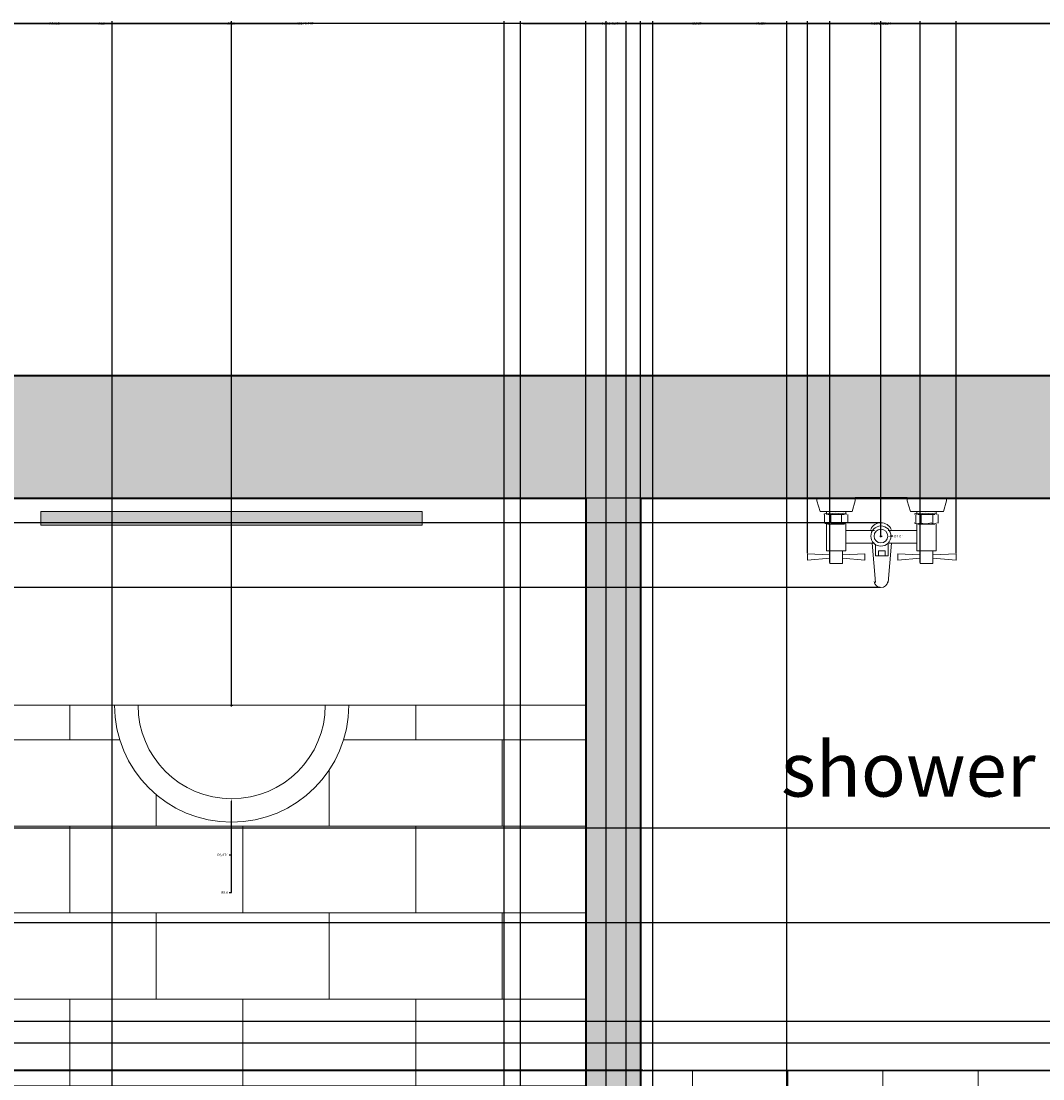
# Model space of a CAD drawing. Units: inches. Extents: x 6 to 575, y 34 to 566.
# Tile 9 of 21: x 76 to 151, y 488 to 566. Entities that reach past the tile are written whole.
import ezdxf

# ---------------------------------------------------------------- set-up
doc = ezdxf.new("R2010")
doc.units = ezdxf.units.IN
for name, color, linetype, lineweight in [('A-ANNO-DIMS', 2, 'Continuous', 18), ('A-ANNO-TEXT', 6, 'Continuous', 18), ('A-FLOR-CASE', 2, 'Continuous', 18), ('A-FLOR-CASE-PATT', 2, 'Continuous', 9), ('A-FLOR-FIXT', 9, 'Continuous', 18), ('A-FLOR-PATT', 252, 'Continuous', 9), ('A-WALL-PATT', 251, 'Continuous', 9), ('FUR', 2, 'Continuous', 18), ('WALLS', 7, 'Continuous', 35)]:
    doc.layers.add(name, color=color, linetype=linetype, lineweight=lineweight)
doc.styles.add('PDF Arial Narrow', font='txt')
doc.styles.get("Standard").update_dxf_attribs({"font": 'arial.ttf'})
doc.dimstyles.get("Standard").update_dxf_attribs({"dimtxt": 0.18, "dimasz": 0.18, "dimexe": 0.18, "dimexo": 0.0625, "dimgap": 0.09, "dimtad": 0, "dimtih": 1, "dimtoh": 1, "dimdec": 4, "dimzin": 0, "dimdsep": 46, "dimtxsty": 'Standard', "dimcen": 0.09, "dimadec": 0, "dimazin": 0, "dimtfac": 1, "dimtdec": 4, "dimtofl": 0, "dimtmove": 0, "dimatfit": 3, "dimfxl": 1, "dimtolj": 1, "dimtzin": 0, "dimarcsym": 0})

# ---------------------------------------------------------------- blocks, each defined once
blk = doc.blocks.new('*D30')
at = {"layer": 'A-ANNO-DIMS', "color": 0, "lineweight": -2, "transparency": 16777216}
for p, q in [((32.596, 539.801), (6.649, 539.801)), ((6.829, 539.621), (6.829, 299.97)), ((6.829, 59.955), (6.829, 299.606)), ((197.625, 59.775), (6.649, 59.775))]:
    blk.add_line(p, q, dxfattribs=at)
at = {"layer": 'A-ANNO-DIMS', "color": 0, "transparency": 16777216}
for points in [[(6.799, 539.621), (6.859, 539.621), (6.829, 539.801)], [(6.799, 59.955), (6.859, 59.955), (6.829, 59.775)]]:
    blk.add_solid(points, dxfattribs=at)
at = {"layer": 'Defpoints', "color": 0, "transparency": 16777216}
for p in [(32.659, 539.801), (6.829, 59.775), (197.687, 59.775)]:
    blk.add_point(p, dxfattribs=at)
at = {"layer": 'A-ANNO-DIMS', "color": 0, "transparency": 16777216, "insert": (6.829, 299.788), "char_height": 0.18, "attachment_point": 5}
blk.add_mtext('\\A1;480', dxfattribs=at)
blk = doc.blocks.new('*D31')
at = {"layer": 'A-ANNO-DIMS', "color": 0, "lineweight": -2, "transparency": 16777216}
for p, q in [((32.659, 539.863), (32.659, 565.811)), ((32.839, 565.631), (96.378, 565.631)), ((160.479, 565.631), (96.939, 565.631)), ((160.659, 539.863), (160.659, 565.811))]:
    blk.add_line(p, q, dxfattribs=at)
at = {"layer": 'A-ANNO-DIMS', "color": 0, "transparency": 16777216}
for points in [[(32.839, 565.661), (32.839, 565.601), (32.659, 565.631)], [(160.479, 565.661), (160.479, 565.601), (160.659, 565.631)]]:
    blk.add_solid(points, dxfattribs=at)
at = {"layer": 'Defpoints', "color": 0, "transparency": 16777216}
for p in [(160.659, 565.631), (32.659, 539.801), (160.659, 539.801)]:
    blk.add_point(p, dxfattribs=at)
at = {"layer": 'A-ANNO-DIMS', "color": 0, "transparency": 16777216, "insert": (96.659, 565.631), "char_height": 0.18, "attachment_point": 5}
blk.add_mtext('\\A1;128', dxfattribs=at)
blk = doc.blocks.new('*D55')
at = {"layer": 'A-ANNO-DIMS', "color": 0, "lineweight": -2, "transparency": 16777216}
for p, q in [((41.659, 286.127), (41.659, 565.811)), ((41.839, 565.631), (81.788, 565.631)), ((122.385, 565.631), (82.436, 565.631)), ((122.565, 286.127), (122.565, 565.811))]:
    blk.add_line(p, q, dxfattribs=at)
at = {"layer": 'A-ANNO-DIMS', "color": 0, "transparency": 16777216}
for points in [[(41.839, 565.661), (41.839, 565.601), (41.659, 565.631)], [(122.385, 565.661), (122.385, 565.601), (122.565, 565.631)]]:
    blk.add_solid(points, dxfattribs=at)
at = {"layer": 'Defpoints', "color": 0, "transparency": 16777216}
for p in [(122.565, 565.631), (41.659, 286.064), (122.565, 286.064)]:
    blk.add_point(p, dxfattribs=at)
at = {"layer": 'A-ANNO-DIMS', "color": 0, "transparency": 16777216, "insert": (82.112, 565.631), "char_height": 0.18, "attachment_point": 5}
blk.add_mtext('\\A1;80.9', dxfattribs=at)
blk = doc.blocks.new('*D62')
at = {"layer": 'A-ANNO-DIMS', "color": 0, "lineweight": -2, "transparency": 16777216}
for p, q in [((117.659, 530.863), (117.659, 565.811)), ((117.839, 565.631), (119.506, 565.631)), ((121.479, 565.631), (119.811, 565.631)), ((121.659, 530.863), (121.659, 565.811))]:
    blk.add_line(p, q, dxfattribs=at)
at = {"layer": 'A-ANNO-DIMS', "color": 0, "transparency": 16777216}
for points in [[(117.839, 565.661), (117.839, 565.601), (117.659, 565.631)], [(121.479, 565.661), (121.479, 565.601), (121.659, 565.631)]]:
    blk.add_solid(points, dxfattribs=at)
at = {"layer": 'Defpoints', "color": 0, "transparency": 16777216}
for p in [(121.659, 565.631), (117.659, 530.801), (121.659, 530.801)]:
    blk.add_point(p, dxfattribs=at)
at = {"layer": 'A-ANNO-DIMS', "color": 0, "transparency": 16777216, "insert": (119.659, 565.631), "char_height": 0.18, "attachment_point": 5}
blk.add_mtext('\\A1;4', dxfattribs=at)
blk = doc.blocks.new('*D66')
at = {"layer": 'A-ANNO-DIMS', "color": 0, "lineweight": -2, "transparency": 16777216}
for p, q in [((41.659, 440.863), (41.659, 565.811)), ((41.839, 565.631), (61.878, 565.631)), ((82.712, 565.631), (62.673, 565.631)), ((82.892, 440.863), (82.892, 565.811))]:
    blk.add_line(p, q, dxfattribs=at)
at = {"layer": 'A-ANNO-DIMS', "color": 0, "transparency": 16777216}
for points in [[(41.839, 565.661), (41.839, 565.601), (41.659, 565.631)], [(82.712, 565.661), (82.712, 565.601), (82.892, 565.631)]]:
    blk.add_solid(points, dxfattribs=at)
at = {"layer": 'Defpoints', "color": 0, "transparency": 16777216}
for p in [(82.892, 565.631), (41.659, 440.801), (82.892, 440.801)]:
    blk.add_point(p, dxfattribs=at)
at = {"layer": 'A-ANNO-DIMS', "color": 0, "transparency": 16777216, "insert": (62.275, 565.631), "char_height": 0.18, "attachment_point": 5}
blk.add_mtext('\\A1;41.23', dxfattribs=at)
blk = doc.blocks.new('*D67')
at = {"layer": 'A-ANNO-DIMS', "color": 0, "lineweight": -2, "transparency": 16777216}
for p, q in [((82.892, 440.863), (82.892, 565.811)), ((83.072, 565.631), (96.81, 565.631)), ((111.479, 565.631), (97.74, 565.631)), ((111.659, 440.863), (111.659, 565.811))]:
    blk.add_line(p, q, dxfattribs=at)
at = {"layer": 'A-ANNO-DIMS', "color": 0, "transparency": 16777216}
for points in [[(83.072, 565.661), (83.072, 565.601), (82.892, 565.631)], [(111.479, 565.661), (111.479, 565.601), (111.659, 565.631)]]:
    blk.add_solid(points, dxfattribs=at)
at = {"layer": 'Defpoints', "color": 0, "transparency": 16777216}
for p in [(111.659, 565.631), (82.892, 440.801), (111.659, 440.801)]:
    blk.add_point(p, dxfattribs=at)
at = {"layer": 'A-ANNO-DIMS', "color": 0, "transparency": 16777216, "insert": (97.275, 565.631), "char_height": 0.18, "attachment_point": 5}
blk.add_mtext('\\A1;28.767', dxfattribs=at)
blk = doc.blocks.new('*D68')
at = {"layer": 'A-ANNO-DIMS', "color": 0, "lineweight": -2, "transparency": 16777216}
for p, q in [((206.596, 530.801), (6.649, 530.801)), ((6.829, 530.621), (6.829, 509.957)), ((6.829, 488.928), (6.829, 509.593)), ((248.571, 488.748), (6.649, 488.748))]:
    blk.add_line(p, q, dxfattribs=at)
at = {"layer": 'A-ANNO-DIMS', "color": 0, "transparency": 16777216}
for points in [[(6.799, 530.621), (6.859, 530.621), (6.829, 530.801)], [(6.799, 488.928), (6.859, 488.928), (6.829, 488.748)]]:
    blk.add_solid(points, dxfattribs=at)
at = {"layer": 'Defpoints', "color": 0, "transparency": 16777216}
for p in [(206.659, 530.801), (6.829, 488.748), (248.633, 488.748)]:
    blk.add_point(p, dxfattribs=at)
at = {"layer": 'A-ANNO-DIMS', "color": 0, "transparency": 16777216, "insert": (6.829, 509.775), "char_height": 0.18, "attachment_point": 5}
blk.add_mtext('\\A1;42.05', dxfattribs=at)
blk = doc.blocks.new('*D71')
at = {"layer": 'A-ANNO-DIMS', "color": 0, "lineweight": -2, "transparency": 16777216}
for p, q in [((246.62, 490.777), (6.649, 490.777)), ((6.829, 490.597), (6.829, 489.945)), ((6.829, 488.928), (6.829, 489.581)), ((248.571, 488.748), (6.649, 488.748))]:
    blk.add_line(p, q, dxfattribs=at)
at = {"layer": 'A-ANNO-DIMS', "color": 0, "transparency": 16777216}
for points in [[(6.799, 490.597), (6.859, 490.597), (6.829, 490.777)], [(6.799, 488.928), (6.859, 488.928), (6.829, 488.748)]]:
    blk.add_solid(points, dxfattribs=at)
at = {"layer": 'Defpoints', "color": 0, "transparency": 16777216}
for p in [(246.683, 490.777), (6.829, 488.748), (248.633, 488.748)]:
    blk.add_point(p, dxfattribs=at)
at = {"layer": 'A-ANNO-DIMS', "color": 0, "transparency": 16777216, "insert": (6.829, 489.763), "char_height": 0.18, "attachment_point": 5}
blk.add_mtext('\\A1;2.03', dxfattribs=at)
blk = doc.blocks.new('*D109')
at = {"layer": 'A-ANNO-DIMS', "color": 0, "lineweight": -2, "transparency": 16777216}
for p, q in [((112.851, 431.863), (112.851, 565.811)), ((113.031, 565.631), (154.931, 565.631)), ((197.479, 565.631), (155.579, 565.631)), ((197.659, 431.863), (197.659, 565.811))]:
    blk.add_line(p, q, dxfattribs=at)
at = {"layer": 'A-ANNO-DIMS', "color": 0, "transparency": 16777216}
for points in [[(113.031, 565.661), (113.031, 565.601), (112.851, 565.631)], [(197.479, 565.661), (197.479, 565.601), (197.659, 565.631)]]:
    blk.add_solid(points, dxfattribs=at)
at = {"layer": 'Defpoints', "color": 0, "transparency": 16777216}
for p in [(197.659, 565.631), (112.851, 431.801), (197.659, 431.801)]:
    blk.add_point(p, dxfattribs=at)
at = {"layer": 'A-ANNO-DIMS', "color": 0, "transparency": 16777216, "insert": (155.255, 565.631), "char_height": 0.18, "attachment_point": 5}
blk.add_mtext('\\A1;84.8', dxfattribs=at)
blk = doc.blocks.new('*D113')
at = {"layer": 'A-ANNO-DIMS', "color": 0, "lineweight": -2, "transparency": 16777216}
for p, q in [((65.649, 530.863), (65.649, 565.811)), ((65.829, 565.631), (91.278, 565.631)), ((117.479, 565.631), (92.03, 565.631)), ((117.659, 530.863), (117.659, 565.811))]:
    blk.add_line(p, q, dxfattribs=at)
at = {"layer": 'A-ANNO-DIMS', "color": 0, "transparency": 16777216}
for points in [[(65.829, 565.661), (65.829, 565.601), (65.649, 565.631)], [(117.479, 565.661), (117.479, 565.601), (117.659, 565.631)]]:
    blk.add_solid(points, dxfattribs=at)
at = {"layer": 'Defpoints', "color": 0, "transparency": 16777216}
for p in [(117.659, 565.631), (65.649, 530.801), (117.659, 530.801)]:
    blk.add_point(p, dxfattribs=at)
at = {"layer": 'A-ANNO-DIMS', "color": 0, "transparency": 16777216, "insert": (91.654, 565.631), "char_height": 0.18, "attachment_point": 5}
blk.add_mtext('\\A1;52.01', dxfattribs=at)
blk = doc.blocks.new('*D118')
at = {"layer": 'A-ANNO-DIMS', "color": 0, "lineweight": -2, "transparency": 16777216}
for p, q in [((65.649, 515.657), (65.649, 565.811)), ((65.829, 565.631), (78.186, 565.631)), ((91.474, 565.631), (79.118, 565.631)), ((91.654, 515.657), (91.654, 565.811))]:
    blk.add_line(p, q, dxfattribs=at)
at = {"layer": 'A-ANNO-DIMS', "color": 0, "transparency": 16777216}
for points in [[(65.829, 565.661), (65.829, 565.601), (65.649, 565.631)], [(91.474, 565.661), (91.474, 565.601), (91.654, 565.631)]]:
    blk.add_solid(points, dxfattribs=at)
at = {"layer": 'Defpoints', "color": 0, "transparency": 16777216}
for p in [(91.654, 565.631), (65.649, 515.594), (91.654, 515.594)]:
    blk.add_point(p, dxfattribs=at)
at = {"layer": 'A-ANNO-DIMS', "color": 0, "transparency": 16777216, "insert": (78.652, 565.631), "char_height": 0.18, "attachment_point": 5}
blk.add_mtext('\\A1;26.005', dxfattribs=at)
blk = doc.blocks.new('*D175')
at = {"layer": 'A-ANNO-DIMS', "color": 0, "lineweight": -2, "transparency": 16777216}
for p, q in [((121.659, 530.863), (121.659, 565.811)), ((121.839, 565.631), (139.387, 565.631)), ((157.689, 565.631), (140.14, 565.631)), ((157.869, 530.898), (157.869, 565.811))]:
    blk.add_line(p, q, dxfattribs=at)
at = {"layer": 'A-ANNO-DIMS', "color": 0, "transparency": 16777216}
for points in [[(121.839, 565.661), (121.839, 565.601), (121.659, 565.631)], [(157.689, 565.661), (157.689, 565.601), (157.869, 565.631)]]:
    blk.add_solid(points, dxfattribs=at)
at = {"layer": 'Defpoints', "color": 0, "transparency": 16777216}
for p in [(157.869, 565.631), (121.659, 530.801), (157.869, 530.836)]:
    blk.add_point(p, dxfattribs=at)
at = {"layer": 'A-ANNO-DIMS', "color": 0, "transparency": 16777216, "insert": (139.764, 565.631), "char_height": 0.18, "attachment_point": 5}
blk.add_mtext('\\A1;36.21', dxfattribs=at)
blk = doc.blocks.new('*D176')
at = {"layer": 'A-ANNO-DIMS', "color": 0, "lineweight": -2, "transparency": 16777216}
for p, q in [((121.596, 530.801), (6.649, 530.801)), ((6.829, 530.621), (6.829, 509.974)), ((6.829, 488.963), (6.829, 509.61)), ((121.839, 488.783), (6.649, 488.783))]:
    blk.add_line(p, q, dxfattribs=at)
at = {"layer": 'A-ANNO-DIMS', "color": 0, "transparency": 16777216}
for points in [[(6.799, 530.621), (6.859, 530.621), (6.829, 530.801)], [(6.799, 488.963), (6.859, 488.963), (6.829, 488.783)]]:
    blk.add_solid(points, dxfattribs=at)
at = {"layer": 'Defpoints', "color": 0, "transparency": 16777216}
for p in [(121.659, 530.801), (6.829, 488.783), (121.902, 488.783)]:
    blk.add_point(p, dxfattribs=at)
at = {"layer": 'A-ANNO-DIMS', "color": 0, "transparency": 16777216, "insert": (6.829, 509.792), "char_height": 0.18, "attachment_point": 5}
blk.add_mtext('\\A1;42.02', dxfattribs=at)
blk = doc.blocks.new('*D177')
at = {"layer": 'A-ANNO-DIMS', "color": 0, "lineweight": -2, "transparency": 16777216}
for p, q in [((139.252, 528.983), (6.649, 528.983)), ((6.829, 528.803), (6.829, 526.786)), ((6.829, 524.404), (6.829, 526.422)), ((139.252, 524.224), (6.649, 524.224))]:
    blk.add_line(p, q, dxfattribs=at)
at = {"layer": 'A-ANNO-DIMS', "color": 0, "transparency": 16777216}
for points in [[(6.799, 528.803), (6.859, 528.803), (6.829, 528.983)], [(6.799, 524.404), (6.859, 524.404), (6.829, 524.224)]]:
    blk.add_solid(points, dxfattribs=at)
at = {"layer": 'Defpoints', "color": 0, "transparency": 16777216}
for p in [(139.314, 528.983), (6.829, 524.224), (139.314, 524.224)]:
    blk.add_point(p, dxfattribs=at)
at = {"layer": 'A-ANNO-DIMS', "color": 0, "transparency": 16777216, "insert": (6.829, 526.604), "char_height": 0.18, "attachment_point": 5}
blk.add_mtext('\\A1;4.759', dxfattribs=at)
blk = doc.blocks.new('*D178')
at = {"layer": 'A-ANNO-DIMS', "color": 0, "lineweight": -2, "transparency": 16777216}
for p, q in [((133.917, 526.763), (133.917, 565.811)), ((134.097, 565.631), (138.923, 565.631)), ((144.659, 565.631), (139.833, 565.631)), ((144.839, 526.763), (144.839, 565.811))]:
    blk.add_line(p, q, dxfattribs=at)
at = {"layer": 'A-ANNO-DIMS', "color": 0, "transparency": 16777216}
for points in [[(134.097, 565.661), (134.097, 565.601), (133.917, 565.631)], [(144.659, 565.661), (144.659, 565.601), (144.839, 565.631)]]:
    blk.add_solid(points, dxfattribs=at)
at = {"layer": 'Defpoints', "color": 0, "transparency": 16777216}
for p in [(144.839, 565.631), (133.917, 526.701), (144.839, 526.701)]:
    blk.add_point(p, dxfattribs=at)
at = {"layer": 'A-ANNO-DIMS', "color": 0, "transparency": 16777216, "insert": (139.378, 565.631), "char_height": 0.18, "attachment_point": 5}
blk.add_mtext('\\A1;10.923', dxfattribs=at)
blk = doc.blocks.new('*D179')
at = {"layer": 'A-ANNO-DIMS', "color": 0, "lineweight": -2, "transparency": 16777216}
for p, q in [((135.555, 526.061), (135.555, 565.811)), ((135.735, 565.631), (138.478, 565.631)), ((142.007, 565.631), (139.264, 565.631)), ((142.187, 526.061), (142.187, 565.811))]:
    blk.add_line(p, q, dxfattribs=at)
at = {"layer": 'A-ANNO-DIMS', "color": 0, "transparency": 16777216}
for points in [[(135.735, 565.661), (135.735, 565.601), (135.555, 565.631)], [(142.007, 565.661), (142.007, 565.601), (142.187, 565.631)]]:
    blk.add_solid(points, dxfattribs=at)
at = {"layer": 'Defpoints', "color": 0, "transparency": 16777216}
for p in [(142.187, 565.631), (135.555, 525.998), (142.187, 525.998)]:
    blk.add_point(p, dxfattribs=at)
at = {"layer": 'A-ANNO-DIMS', "color": 0, "transparency": 16777216, "insert": (138.871, 565.631), "char_height": 0.18, "attachment_point": 5}
blk.add_mtext('\\A1;6.632', dxfattribs=at)
blk = doc.blocks.new('*D180')
at = {"layer": 'A-ANNO-DIMS', "color": 0, "lineweight": -2, "transparency": 16777216}
for p, q in [((121.659, 530.863), (121.659, 565.811)), ((121.839, 565.631), (130.031, 565.631)), ((139.134, 565.631), (130.942, 565.631)), ((139.314, 528.071), (139.314, 565.811))]:
    blk.add_line(p, q, dxfattribs=at)
at = {"layer": 'A-ANNO-DIMS', "color": 0, "transparency": 16777216}
for points in [[(121.839, 565.661), (121.839, 565.601), (121.659, 565.631)], [(139.134, 565.661), (139.134, 565.601), (139.314, 565.631)]]:
    blk.add_solid(points, dxfattribs=at)
at = {"layer": 'Defpoints', "color": 0, "transparency": 16777216}
for p in [(139.314, 565.631), (121.659, 530.801), (139.314, 528.008)]:
    blk.add_point(p, dxfattribs=at)
at = {"layer": 'A-ANNO-DIMS', "color": 0, "transparency": 16777216, "insert": (130.486, 565.631), "char_height": 0.18, "attachment_point": 5}
blk.add_mtext('\\A1;17.656', dxfattribs=at)
blk = doc.blocks.new('*D181')
at = {"layer": 'A-ANNO-DIMS', "color": 0, "lineweight": -2, "transparency": 16777216}
for p, q in [((197.596, 530.801), (6.649, 530.801)), ((6.829, 530.621), (6.829, 515.387)), ((6.829, 499.788), (6.829, 515.023)), ((170.657, 499.608), (6.649, 499.608))]:
    blk.add_line(p, q, dxfattribs=at)
at = {"layer": 'A-ANNO-DIMS', "color": 0, "transparency": 16777216}
for points in [[(6.799, 530.621), (6.859, 530.621), (6.829, 530.801)], [(6.799, 499.788), (6.859, 499.788), (6.829, 499.608)]]:
    blk.add_solid(points, dxfattribs=at)
at = {"layer": 'Defpoints', "color": 0, "transparency": 16777216}
for p in [(197.659, 530.801), (6.829, 499.608), (170.719, 499.608)]:
    blk.add_point(p, dxfattribs=at)
at = {"layer": 'A-ANNO-DIMS', "color": 0, "transparency": 16777216, "insert": (6.829, 515.205), "char_height": 0.18, "attachment_point": 5}
blk.add_mtext('\\A1;31.19', dxfattribs=at)
blk = doc.blocks.new('*D183')
at = {"layer": 'A-ANNO-DIMS', "color": 0, "lineweight": -2, "transparency": 16777216}
for p, q in [((181.056, 506.572), (6.649, 506.572)), ((6.829, 506.392), (6.829, 499.652)), ((6.829, 492.552), (6.829, 499.291)), ((180.432, 492.372), (6.649, 492.372))]:
    blk.add_line(p, q, dxfattribs=at)
at = {"layer": 'A-ANNO-DIMS', "color": 0, "transparency": 16777216}
for points in [[(6.799, 506.392), (6.859, 506.392), (6.829, 506.572)], [(6.799, 492.552), (6.859, 492.552), (6.829, 492.372)]]:
    blk.add_solid(points, dxfattribs=at)
at = {"layer": 'Defpoints', "color": 0, "transparency": 16777216}
for p in [(6.829, 506.572), (181.118, 506.572), (180.494, 492.372)]:
    blk.add_point(p, dxfattribs=at)
at = {"layer": 'A-ANNO-DIMS', "color": 0, "transparency": 16777216, "insert": (6.829, 499.472), "char_height": 0.18, "attachment_point": 5}
blk.add_mtext('\\A1;14.2', dxfattribs=at)
blk = doc.blocks.new('*D200')
at = {"layer": 'A-ANNO-DIMS', "color": 0, "lineweight": -2, "transparency": 16777216}
for p, q in [((119.133, 448.153), (119.133, 565.811)), ((119.313, 565.631), (125.311, 565.631)), ((132.22, 565.631), (126.221, 565.631)), ((132.4, 471.132), (132.4, 565.811))]:
    blk.add_line(p, q, dxfattribs=at)
at = {"layer": 'A-ANNO-DIMS', "color": 0, "transparency": 16777216}
for points in [[(119.313, 565.661), (119.313, 565.601), (119.133, 565.631)], [(132.22, 565.661), (132.22, 565.601), (132.4, 565.631)]]:
    blk.add_solid(points, dxfattribs=at)
at = {"layer": 'Defpoints', "color": 0, "transparency": 16777216}
for p in [(132.4, 565.631), (132.4, 471.07), (119.133, 448.091)]:
    blk.add_point(p, dxfattribs=at)
at = {"layer": 'A-ANNO-DIMS', "color": 0, "transparency": 16777216, "insert": (125.766, 565.631), "char_height": 0.18, "attachment_point": 5}
blk.add_mtext('\\A1;13.267', dxfattribs=at)
blk = doc.blocks.new('*D202')
at = {"layer": 'A-ANNO-DIMS', "color": 0, "lineweight": -2, "transparency": 16777216}
for p, q in [((117.659, 446.863), (117.659, 565.811)), ((117.839, 565.631), (118.737, 565.631)), ((120.427, 565.631), (119.528, 565.631)), ((120.607, 446.863), (120.607, 565.811))]:
    blk.add_line(p, q, dxfattribs=at)
at = {"layer": 'A-ANNO-DIMS', "color": 0, "transparency": 16777216}
for points in [[(117.839, 565.661), (117.839, 565.601), (117.659, 565.631)], [(120.427, 565.661), (120.427, 565.601), (120.607, 565.631)]]:
    blk.add_solid(points, dxfattribs=at)
at = {"layer": 'Defpoints', "color": 0, "transparency": 16777216}
for p in [(120.607, 565.631), (117.659, 446.801), (120.607, 446.801)]:
    blk.add_point(p, dxfattribs=at)
at = {"layer": 'A-ANNO-DIMS', "color": 0, "transparency": 16777216, "insert": (119.133, 565.631), "char_height": 0.18, "attachment_point": 5}
blk.add_mtext('\\A1;2.948', dxfattribs=at)
blk = doc.blocks.new('*D205')
at = {"layer": 'A-ANNO-DIMS', "color": 0, "lineweight": -2, "transparency": 16777216}
for p, q in [((119.133, 447.601), (119.133, 565.811)), ((119.313, 565.631), (119.485, 565.631)), ((120.427, 565.631), (120.255, 565.631)), ((120.607, 447.601), (120.607, 565.811))]:
    blk.add_line(p, q, dxfattribs=at)
at = {"layer": 'A-ANNO-DIMS', "color": 0, "transparency": 16777216}
for points in [[(119.313, 565.661), (119.313, 565.601), (119.133, 565.631)], [(120.427, 565.661), (120.427, 565.601), (120.607, 565.631)]]:
    blk.add_solid(points, dxfattribs=at)
at = {"layer": 'Defpoints', "color": 0, "transparency": 16777216}
for p in [(120.607, 565.631), (119.133, 447.538), (120.607, 447.538)]:
    blk.add_point(p, dxfattribs=at)
at = {"layer": 'A-ANNO-DIMS', "color": 0, "transparency": 16777216, "insert": (119.87, 565.631), "char_height": 0.18, "attachment_point": 5}
blk.add_mtext('\\A1;1.474', dxfattribs=at)
blk = doc.blocks.new('*D239')
at = {"layer": 'A-ANNO-DIMS', "color": 0, "lineweight": -2, "transparency": 16777216}
for p, q in [((91.654, 515.504), (91.654, 515.684)), ((91.564, 515.594), (91.744, 515.594)), ((91.654, 501.835), (91.654, 506.815)), ((91.474, 501.835), (91.654, 501.835))]:
    blk.add_line(p, q, dxfattribs=at)
at = {"layer": 'A-ANNO-DIMS', "color": 0, "transparency": 16777216}
blk.add_solid([(91.624, 506.815), (91.684, 506.815), (91.654, 506.995)], dxfattribs=at)
at = {"layer": 'Defpoints', "color": 0, "transparency": 16777216}
for p in [(91.654, 515.594), (91.654, 506.995)]:
    blk.add_point(p, dxfattribs=at)
at = {"layer": 'A-ANNO-DIMS', "color": 0, "transparency": 16777216, "insert": (91.134, 501.835), "char_height": 0.18, "attachment_point": 5}
blk.add_mtext('\\A1;R8.6', dxfattribs=at)
blk = doc.blocks.new('*D240')
at = {"layer": 'A-ANNO-DIMS', "color": 0, "lineweight": -2, "transparency": 16777216}
for p, q in [((91.654, 515.504), (91.654, 515.684)), ((91.564, 515.594), (91.744, 515.594)), ((91.654, 504.596), (91.654, 508.54)), ((91.474, 504.596), (91.654, 504.596))]:
    blk.add_line(p, q, dxfattribs=at)
at = {"layer": 'A-ANNO-DIMS', "color": 0, "transparency": 16777216}
blk.add_solid([(91.624, 508.54), (91.684, 508.54), (91.654, 508.72)], dxfattribs=at)
at = {"layer": 'Defpoints', "color": 0, "transparency": 16777216}
for p in [(91.654, 515.594), (91.654, 508.72)]:
    blk.add_point(p, dxfattribs=at)
at = {"layer": 'A-ANNO-DIMS', "color": 0, "transparency": 16777216, "insert": (90.995, 504.596), "char_height": 0.18, "attachment_point": 5}
blk.add_mtext('\\A1;R6.874', dxfattribs=at)
blk = doc.blocks.new('*D251')
at = {"layer": 'A-ANNO-DIMS', "color": 0, "lineweight": -2, "transparency": 16777216}
for p, q in [((139.314, 527.918), (139.314, 528.098)), ((139.224, 528.008), (139.404, 528.008)), ((140.181, 527.994), (140.001, 527.997))]:
    blk.add_line(p, q, dxfattribs=at)
at = {"layer": 'A-ANNO-DIMS', "color": 0, "transparency": 16777216}
blk.add_solid([(140.002, 528.027), (140.001, 527.967), (139.821, 528)], dxfattribs=at)
at = {"layer": 'Defpoints', "color": 0, "transparency": 16777216}
for p in [(138.807, 528.016), (139.821, 528)]:
    blk.add_point(p, dxfattribs=at)
at = {"layer": 'A-ANNO-DIMS', "color": 0, "transparency": 16777216, "insert": (140.586, 527.994), "char_height": 0.18, "attachment_point": 5}
blk.add_mtext('\\A1;∅1.01', dxfattribs=at)

msp = doc.modelspace()

# ---------------------------------------------------------------- hatches: boundary and pattern name
at = {"layer": 'A-FLOR-CASE-PATT'}
h = msp.add_hatch(color=256, dxfattribs=at)
h.dxf.hatch_style = 1
h.paths.add_polyline_path([(105.6494, 529.801), (77.6494, 529.801), (77.6494, 528.801), (105.6494, 528.801)])
at = {"layer": 'A-FLOR-PATT'}
h = msp.add_hatch(dxfattribs=at)
h.set_pattern_fill('ANGLE', color=256)
h.set_pattern_definition([(0, (-98.035, 170.1465), (0, 6.985), [5.08, -1.905]), (90, (-98.035, 170.1465), (-6.985, 4e-16), [5.08, -1.905])])
edge = h.paths.add_edge_path()
edge.add_line((191.6511, 494.1664), (190.4028, 493.9036))
edge.add_line((190.4028, 493.9036), (189.6226, 493.6983))
edge.add_line((189.6226, 493.6983), (188.2183, 493.3862))
edge.add_line((188.2183, 493.3862), (187.2685, 493.2437))
edge.add_line((187.2685, 493.2437), (187.204, 493.2302))
edge.add_line((187.204, 493.2302), (187.0709, 493.2141))
edge.add_line((187.0709, 493.2141), (185.0975, 492.9181))
edge.add_line((185.0975, 492.9181), (185.0904, 492.9751))
edge.add_line((185.0904, 492.9751), (183.6001, 492.7952))
edge.add_line((183.6001, 492.7952), (183.5371, 492.7621))
edge.add_line((183.5371, 492.7621), (181.5041, 492.4232))
edge.add_spline(control_points=[(181.5178, 492.4356), (181.2536, 492.4138), (180.9898, 492.4), (180.727, 492.3941)], knot_values=[2.9292163, 2.9292163, 2.9292163, 2.9292163, 3, 3, 3, 3], degree=3, periodic=0)
edge.add_line((180.727, 492.3941), (180.4943, 492.372))
edge.add_line((180.4943, 492.372), (180.175, 492.3932))
edge.add_spline(control_points=[(180.175, 492.3932), (179.0187, 492.4156), (177.8901, 492.5895), (176.8377, 492.8977)], knot_values=[2.5659353, 2.5659353, 2.5659353, 2.5659353, 2.8794912, 2.8794912, 2.8794912, 2.8794912], degree=3, periodic=0)
edge.add_line((176.8377, 492.8977), (176.5264, 492.9696))
edge.add_spline(control_points=[(176.656, 492.9525), (176.2658, 493.0735), (175.8866, 493.2132), (175.521, 493.3707)], knot_values=[2.4305318, 2.4305318, 2.4305318, 2.4305318, 2.5478122, 2.5478122, 2.5478122, 2.5478122], degree=3, periodic=0)
edge.add_line((175.521, 493.3707), (175.267, 493.4642))
edge.add_line((175.267, 493.4642), (175.098, 493.5637))
edge.add_spline(control_points=[(175.098, 493.5637), (173.9351, 494.1251), (172.9292, 494.8734), (172.1696, 495.7766)], knot_values=[2, 2, 2, 2, 2.3846171, 2.3846171, 2.3846171, 2.3846171], degree=3, periodic=0)
edge.add_line((172.9656, 494.9581), (172.8363, 495.1004))
edge.add_spline(control_points=[(175.098, 493.5637), (173.9351, 494.1251), (172.9292, 494.8734), (172.1696, 495.7766)], knot_values=[2, 2, 2, 2, 2.3846171, 2.3846171, 2.3846171, 2.3846171], degree=3, periodic=0)
edge.add_line((171.9925, 495.9563), (171.8762, 496.1888))
edge.add_spline(control_points=[(172.1696, 495.7766), (170.1947, 498.1251), (170.2393, 501.0999), (172.2842, 503.4158)], knot_values=[1, 1, 1, 1, 2, 2, 2, 2], degree=3, periodic=0)
edge.add_line((170.6556, 499.1388), (170.6881, 499.323))
edge.add_spline(control_points=[(172.1696, 495.7766), (170.1947, 498.1251), (170.2393, 501.0999), (172.2842, 503.4158)], knot_values=[1, 1, 1, 1, 2, 2, 2, 2], degree=3, periodic=0)
edge.add_spline(control_points=[(172.2842, 503.4158), (174.3291, 505.7317), (178.0076, 506.9734), (181.7304, 506.6045)], knot_values=[0, 0, 0, 0, 1, 1, 1, 1], degree=3, periodic=0)
edge.add_line((174.0548, 504.9343), (174.2554, 505.022))
edge.add_spline(control_points=[(172.2842, 503.4158), (174.3291, 505.7317), (178.0076, 506.9734), (181.7304, 506.6045)], knot_values=[0, 0, 0, 0, 1, 1, 1, 1], degree=3, periodic=0)
edge.add_line((178.4031, 506.5313), (178.1947, 506.4718))
edge.add_spline(control_points=[(172.2842, 503.4158), (174.3291, 505.7317), (178.0076, 506.9734), (181.7304, 506.6045)], knot_values=[0, 0, 0, 0, 1, 1, 1, 1], degree=3, periodic=0)
edge.add_line((181.5796, 506.6123), (181.6459, 506.5957))
edge.add_arc((179.34, 495.0824), 11.742, 73.636084, 78.674278, ccw=False)
edge.add_arc((178.5598, 454.8227), 51.688, 83.52982, 85.463383, ccw=False)
edge.add_line((184.3843, 506.1814), (184.5513, 506.1814))
edge.add_line((184.5513, 506.1814), (184.7887, 506.134))
edge.add_arc((178.5598, 454.8227), 51.688, 75.328548, 83.07845, ccw=False)
edge.add_line((191.6511, 504.8253), (191.6511, 530.801))
edge.add_line((191.6511, 530.801), (184.6586, 530.801))
edge.add_line((184.6586, 530.801), (160.6586, 530.801))
edge.add_line((160.6586, 530.801), (157.8686, 530.801))
edge.add_line((157.8686, 530.801), (157.8686, 488.7831))
edge.add_line((157.8686, 488.7831), (121.6586, 488.7831))
edge.add_line((121.6586, 488.7831), (121.6586, 474.801))
edge.add_line((121.6586, 474.801), (120.6068, 474.801))
edge.add_line((120.6068, 474.801), (120.6068, 474.0666))
edge.add_arc((120.0902, 447.538), 26.5336, 62.388015, 88.884314, ccw=False)
edge.add_line((132.388, 471.0496), (132.3995, 471.0696))
edge.add_line((132.3995, 471.0696), (133.357, 470.5168))
edge.add_line((133.357, 470.5168), (120.0902, 447.538))
edge.add_line((120.0902, 447.538), (120.6068, 447.538))
edge.add_line((120.6068, 447.538), (121.6586, 446.801))
edge.add_line((121.6586, 446.801), (121.6586, 440.801))
edge.add_line((121.6586, 440.801), (176.6714, 440.801))
edge.add_line((176.6714, 440.801), (176.6714, 470.8385))
edge.add_line((176.6714, 470.8385), (191.6511, 470.8385))
edge.add_line((191.6511, 470.8385), (191.6511, 494.1664))
h = msp.add_hatch(dxfattribs=at)
h.set_pattern_fill('BRICK', color=256)
h.set_pattern_definition([(0, (-98.035, 170.1465), (0, 6.35), []), (90, (-98.035, 170.147), (-12.7, 8e-16), [6.35, -6.35]), (90, (-91.685, 170.147), (-12.7, 8e-16), [-6.35, 6.35])])
h.paths.add_polyline_path([(180.8711, 269.7588), (182.4439, 270.6668), (182.4628, 270.6341, -0.1161983), (201.8275, 275.5902), (201.8275, 276.801), (197.6586, 276.801), (197.6586, 293.1641), (182.6401, 293.1641), (182.6401, 348.324), (197.6586, 348.324), (197.6586, 407.7709), (112.8513, 407.7709), (112.8513, 431.801), (111.6586, 431.801), (111.6586, 440.801), (117.6586, 440.801), (117.6586, 446.801), (117.6586, 448.2751), (117.6586, 473.3269), (117.6586, 474.801), (117.6586, 515.5941), (100.2533, 515.5941, -1), (83.0548, 515.5941), (65.6494, 515.5941), (65.6494, 440.801), (82.8918, 440.801), (82.8918, 431.801), (82.8918, 407.7709), (41.6586, 407.7709), (41.6586, 379.0637), (62.6459, 379.0637), (62.6459, 358.0764), (122.565, 358.0764), (122.565, 286.0643), (62.6459, 286.0643), (62.6459, 265.077), (41.6586, 265.077), (41.6586, 224.801), (41.6586, 212.801), (71.6586, 212.801), (167.6586, 212.801), (197.6586, 212.801), (197.6586, 230.801), (201.8157, 230.801), (201.8157, 233.4817)])
h.paths.add_polyline_path([(133.3414, 245.1275), (133.3317, 245.1352), (133.3317, 245.104)], flags=16)
h.paths.add_polyline_path([(133.3317, 222.1662), (85.3496, 222.1662), (85.3496, 243.7443, -0.5009073), (87.1831, 246.1963), (107.4292, 246.1963), (111.2522, 246.1963), (131.4202, 246.1963, -0.4142136), (133.3317, 244.2848)], flags=16)
h.paths.add_polyline_path([(72.7105, 244.4018), (72.7105, 220.3718), (48.6804, 220.3718), (48.6804, 244.4018)], flags=16)
h.paths.add_polyline_path([(71.7466, 237.8955, -1), (59.8096, 237.8955, -1)], flags=0)
at = {"layer": 'A-WALL-PATT'}
h = msp.add_hatch(color=256, dxfattribs=at)
h.dxf.hatch_style = 1
h.paths.add_polyline_path([(160.6586, 539.801), (32.6586, 539.801), (32.6586, 272.801), (41.6586, 272.801), (41.6586, 286.0643), (41.6586, 358.0764), (41.6586, 379.0637), (41.6586, 407.7709), (41.6194, 407.7709), (41.6194, 431.801), (82.8918, 431.801), (82.8918, 440.801), (65.6494, 440.801), (65.6494, 440.7732), (41.6194, 440.7732), (41.6194, 515.5941), (41.6586, 530.801), (117.6586, 530.801), (117.6586, 474.801), (120.6068, 474.801), (121.6586, 474.801), (121.6586, 530.801), (137.4275, 530.801), (137.4275, 530.8356), (141.2505, 530.8356), (160.6586, 530.801)])
h.paths.add_polyline_path([(71.6586, 212.801), (41.6586, 212.801), (41.6586, 224.801), (32.6586, 224.801), (32.6586, 203.801), (71.6586, 203.801)])
h.paths.add_polyline_path([(206.6586, 215.801), (246.6586, 215.801), (246.6586, 224.801), (206.6586, 224.801), (206.6586, 230.801), (201.8157, 230.801), (197.6586, 230.801), (197.6586, 212.801), (167.6586, 212.801), (167.6586, 203.801), (206.6586, 203.801)])
h.paths.add_polyline_path([(383.6586, 224.801), (334.6586, 224.801), (334.6586, 215.801), (374.6586, 215.801), (374.6586, 203.801), (384.0753, 203.801), (407.6586, 203.801), (407.6586, 212.801), (383.6586, 212.801)])
h.paths.add_polyline_path([(548.6586, 270.801), (539.6586, 270.801), (539.6586, 212.801), (515.6586, 212.801), (515.6586, 203.801), (548.6586, 203.801)])
h.paths.add_polyline_path([(548.6586, 412.801), (545.7108, 412.801), (539.6586, 412.801), (539.6586, 382.801), (433.708, 382.801), (433.708, 378.801), (539.6586, 378.801), (539.6586, 366.801), (548.6586, 366.801)])
h.paths.add_polyline_path([(548.6586, 539.801), (455.9436, 539.801), (455.9436, 530.801), (539.6586, 530.801), (539.6586, 440.801), (548.6586, 440.801)])
h.paths.add_polyline_path([(407.9436, 539.801), (362.6586, 539.801), (362.6586, 530.801), (374.6586, 530.801), (374.6586, 452.801), (354.6586, 452.801), (354.6586, 448.801), (374.6586, 448.801), (374.6586, 278.801), (383.6586, 278.801), (383.6586, 530.801), (407.9436, 530.801)])
h.paths.add_polyline_path([(338.6586, 539.801), (320.6586, 539.801), (320.6586, 530.801), (322.6586, 530.801), (322.6586, 448.801), (326.6586, 448.801), (326.6586, 530.801), (338.6586, 530.801)])
h.paths.add_polyline_path([(272.6586, 539.801), (184.6586, 539.801), (184.6586, 530.801), (197.6586, 530.801), (197.6586, 440.801), (176.6714, 440.801), (121.6586, 440.801), (121.6586, 446.801), (117.6586, 446.801), (117.6586, 440.801), (111.6586, 440.801), (111.6586, 431.801), (197.6586, 431.801), (197.6586, 407.7709), (197.6586, 276.801), (206.6586, 276.801), (206.6586, 530.801), (272.6586, 530.801)])

# ---------------------------------------------------------------- linework, layer by layer
at = {"layer": 'A-FLOR-CASE'}
msp.add_line((41.6194, 515.5941), (117.6586, 515.5941), dxfattribs=at)
msp.add_lwpolyline([(77.6494, 529.801), (105.6494, 529.801), (105.6494, 528.801), (77.6494, 528.801)], close=True, dxfattribs=at)
at = {"layer": 'A-FLOR-FIXT'}
for points in [[(121.9016, 488.7831), (157.8686, 488.7831), (157.8686, 530.8356)], [(144.1372, 530.8356), (144.1372, 530.6016), (143.9031, 529.8214), (141.4845, 529.8214), (141.2505, 530.6016), (141.2505, 530.8356), (137.4275, 530.8356), (137.4275, 530.6016), (137.1934, 529.8214), (134.8528, 529.8214), (134.6188, 530.6016), (134.6188, 530.8356)], [(135.321, 529.8214), (135.321, 529.5873)], [(136.7253, 529.8214), (136.7253, 529.5873)], [(141.9526, 529.8214), (141.9526, 529.5873)], [(143.357, 529.8214), (143.357, 529.5873)], [(135.1649, 528.9632), (135.1649, 529.5873)], [(135.321, 528.8851), (135.321, 526.9347), (136.7253, 526.9347), (136.7253, 528.8851)], [(135.399, 529.5873), (136.6473, 529.5873)], [(136.6473, 528.8851), (135.399, 528.8851)], [(135.555, 528.8851), (136.4913, 528.8851)], [(135.633, 528.9632), (135.633, 529.5873)], [(136.4132, 528.9632), (136.4132, 529.5873)], [(136.8814, 529.5873), (136.8814, 528.9632)], [(141.8746, 529.5873), (141.8746, 528.9632)], [(143.357, 528.8851), (143.357, 526.9347), (141.9526, 526.9347), (141.9526, 528.8851)], [(143.279, 529.5873), (142.0307, 529.5873)], [(142.0307, 528.8851), (143.279, 528.8851)], [(143.1229, 528.8851), (142.1867, 528.8851)], [(142.2647, 528.9632), (142.2647, 529.5873)], [(143.1229, 528.9632), (143.1229, 529.5873)], [(143.513, 528.9632), (143.513, 529.5873)], [(138.8318, 528.417), (136.7253, 528.417)], [(141.9526, 528.417), (139.8461, 528.417)], [(138.8318, 527.4808), (136.7253, 527.4808)], [(138.6758, 527.4808), (138.9099, 524.5941)], [(139.8461, 527.4028), (139.8461, 526.5446), (138.9099, 526.5446), (138.9099, 527.4028)], [(141.9526, 527.4808), (139.8461, 527.4808)], [(140.0802, 527.4808), (139.8461, 524.5941)], [(135.555, 526.6226), (133.9166, 526.7006), (133.9166, 526.2325), (135.555, 526.3885)], [(135.555, 526.9347), (135.555, 525.9984), (136.4913, 525.9984), (136.4913, 526.9347)], [(136.4913, 526.6226), (138.1297, 526.7006), (138.1297, 526.2325), (136.4913, 526.3885)], [(139.1439, 526.5446), (139.1439, 526.9347), (139.612, 526.9347), (139.612, 526.5446)], [(142.1867, 526.6226), (140.5483, 526.7006), (140.5483, 526.2325), (142.1867, 526.3885)], [(143.1229, 526.9347), (143.1229, 525.9984), (142.1867, 525.9984), (142.1867, 526.9347)], [(143.1229, 526.6226), (144.8394, 526.7006), (144.8394, 526.2325), (143.1229, 526.3885)]]:
    msp.add_lwpolyline(points, dxfattribs=at)
for points in [[(136.8044, 529.6243, 0.2771486), (136.373, 529.6281, 0.1385508), (135.5457, 529.6281, 0.2771486), (135.1142, 529.6243)], [(143.4363, 529.6243, 0.2771486), (143.0049, 529.6281, 0.1385508), (142.1776, 529.6281, 0.2771486), (141.7462, 529.6243)], [(135.1142, 528.9665, 0.2771486), (135.556, 528.9665, 0.1385508), (136.373, 528.9627, 0.2771486), (136.8044, 528.9665)], [(141.7462, 528.9665, 0.2771486), (142.1776, 528.9627, 0.1385508), (142.9945, 528.9665, 0.2771486), (143.4363, 528.9665)]]:
    msp.add_lwpolyline(points, format="xyb", dxfattribs=at)
for radius in [0.7412, 0.5071]:
    msp.add_circle((139.3143, 528.008), radius, dxfattribs=at)
for centre, radius, start, end in [((139.3143, 528.1641), 0.8192, 23.966665, 156.033335), ((139.3143, 524.7311), 0.5071, 187.108129, 352.891871)]:
    msp.add_arc(centre, radius, start, end, dxfattribs=at)
at = {"layer": 'FUR'}
for radius in [8.5992, 6.8736]:
    msp.add_arc((91.654, 515.5941), radius, 180, 0, dxfattribs=at)
at = {"layer": 'WALLS'}
for p, q in [((32.6586, 539.801), (160.6586, 539.801)), ((41.6586, 530.801), (117.6586, 530.801)), ((117.6586, 530.801), (117.6586, 474.801)), ((121.6586, 530.801), (121.6586, 474.801)), ((121.6586, 530.801), (160.6586, 530.801))]:
    msp.add_line(p, q, dxfattribs=at)

# ---------------------------------------------------------------- texts
at = {"layer": 'A-ANNO-TEXT', "insert": (131.9761, 510.3622), "char_height": 4.00034, "attachment_point": 4, "style": 'PDF Arial Narrow'}
msp.add_mtext('shower', dxfattribs=at)

# ---------------------------------------------------------------- dimensions: what is measured, and where the dimension line sits
at = {"layer": 'A-ANNO-DIMS'}
for base, p1, p2, override, picture, middle in [((160.6586, 565.631), (32.6586, 539.801), (160.6586, 539.801), {"dimdec": 0, "dimlfac": 1, "dimrnd": 0, "dimzin": 0, "dimdsep": 46, "dimlunit": 2}, '*D31', (96.6586, 565.631)), ((122.565, 565.631), (41.6586, 286.0643), (122.565, 286.0643), {"dimdec": 1, "dimlfac": 1, "dimrnd": 0, "dimzin": 0, "dimdsep": 46, "dimlunit": 2}, '*D55', (82.1118, 565.631)), ((82.8918, 565.631), (41.6586, 440.801), (82.8918, 440.801), {"dimdec": 2, "dimlfac": 1, "dimrnd": 0, "dimzin": 0, "dimdsep": 46, "dimlunit": 2}, '*D66', (62.2752, 565.631)), ((117.6586, 565.631), (65.6494, 530.801), (117.6586, 530.801), {"dimdec": 2, "dimlfac": 1, "dimrnd": 0, "dimzin": 0, "dimdsep": 46, "dimlunit": 2}, '*D113', (91.654, 565.631)), ((91.654, 565.631), (65.6494, 515.5941), (91.654, 515.5941), {"dimdec": 3, "dimlfac": 1, "dimrnd": 0, "dimzin": 0, "dimdsep": 46, "dimlunit": 2}, '*D118', (78.6517, 565.631)), ((111.6586, 565.631), (82.8918, 440.801), (111.6586, 440.801), {"dimdec": 3, "dimlfac": 1, "dimrnd": 0, "dimzin": 0, "dimdsep": 46, "dimlunit": 2}, '*D67', (97.2752, 565.631)), ((197.6586, 565.631), (112.8513, 431.801), (197.6586, 431.801), {"dimdec": 1, "dimlfac": 1, "dimrnd": 0, "dimzin": 0, "dimdsep": 46, "dimlunit": 2}, '*D109', (155.255, 565.631)), ((121.6586, 565.631), (117.6586, 530.801), (121.6586, 530.801), {"dimdec": 0, "dimlfac": 1, "dimrnd": 0, "dimzin": 0, "dimdsep": 46, "dimlunit": 2}, '*D62', (119.6586, 565.631)), ((120.6068, 565.631), (117.6586, 446.801), (120.6068, 446.801), {"dimdec": 3, "dimlfac": 1, "dimrnd": 0, "dimzin": 0, "dimdsep": 46, "dimlunit": 2}, '*D202', (119.1327, 565.631)), ((132.3995, 565.631), (119.1327, 448.0908), (132.3995, 471.0696), {"dimdec": 3, "dimlfac": 1, "dimrnd": 0, "dimzin": 0, "dimdsep": 46, "dimlunit": 2}, '*D200', (125.7661, 565.631)), ((120.6068, 565.631), (119.1327, 447.538), (120.6068, 447.538), {"dimdec": 3, "dimlfac": 1, "dimrnd": 0, "dimzin": 0, "dimdsep": 46, "dimlunit": 2}, '*D205', (119.8698, 565.631)), ((157.8686, 565.631), (121.6586, 530.801), (157.8686, 530.8356), {"dimdec": 2, "dimlfac": 1, "dimrnd": 0, "dimzin": 0, "dimdsep": 46, "dimlunit": 2}, '*D175', (139.7636, 565.631)), ((139.3143, 565.631), (121.6586, 530.801), (139.3143, 528.008), {"dimdec": 3, "dimlfac": 1, "dimrnd": 0, "dimzin": 0, "dimdsep": 46, "dimlunit": 2}, '*D180', (130.4865, 565.631)), ((144.8394, 565.631), (133.9166, 526.7006), (144.8394, 526.7006), {"dimdec": 3, "dimlfac": 1, "dimrnd": 0, "dimzin": 0, "dimdsep": 46, "dimlunit": 2}, '*D178', (139.378, 565.631)), ((142.1867, 565.631), (135.555, 525.9984), (142.1867, 525.9984), {"dimdec": 3, "dimlfac": 1, "dimrnd": 0, "dimzin": 0, "dimdsep": 46, "dimlunit": 2}, '*D179', (138.8709, 565.631))]:
    dim = msp.add_linear_dim(base=base, p1=p1, p2=p2, dimstyle='Standard', override=override, dxfattribs=at)
    dim.commit()
    dim.dimension.update_dxf_attribs({"geometry": picture, "text_midpoint": middle})
for base, p1, p2, override, picture, middle in [((6.8286, 59.7747), (32.6586, 539.801), (197.6872, 59.7747), {"dimdec": 0, "dimlfac": 1, "dimrnd": 0, "dimzin": 0, "dimdsep": 46, "dimlunit": 2}, '*D30', (6.8286, 299.7878)), ((6.8286, 488.7484), (206.6586, 530.801), (248.6332, 488.7484), {"dimdec": 2, "dimlfac": 1, "dimrnd": 0, "dimzin": 0, "dimdsep": 46, "dimlunit": 2}, '*D68', (6.8286, 509.7747)), ((6.8286, 488.7831), (121.6586, 530.801), (121.9016, 488.7831), {"dimdec": 2, "dimlfac": 1, "dimrnd": 0, "dimzin": 0, "dimdsep": 46, "dimlunit": 2}, '*D176', (6.8286, 509.792)), ((6.8286, 499.6084), (197.6586, 530.801), (170.7195, 499.6084), {"dimdec": 2, "dimlfac": 1, "dimrnd": 0, "dimzin": 0, "dimdsep": 46, "dimlunit": 2}, '*D181', (6.8286, 515.2047)), ((6.8286, 524.224), (139.3143, 528.9833), (139.3143, 524.224), {"dimdec": 3, "dimlfac": 1, "dimrnd": 0, "dimzin": 0, "dimdsep": 46, "dimlunit": 2}, '*D177', (6.8286, 526.6036)), ((6.8286, 506.5715), (180.4943, 492.372), (181.1185, 506.5715), {"dimdec": 1, "dimlfac": 1, "dimrnd": 0, "dimzin": 0, "dimdsep": 46, "dimlunit": 2}, '*D183', (6.8286, 499.4717)), ((6.8286, 488.7484), (246.6827, 490.7769), (248.6332, 488.7484), {"dimdec": 2, "dimlfac": 1, "dimrnd": 0, "dimzin": 0, "dimdsep": 46, "dimlunit": 2}, '*D71', (6.8286, 489.7627))]:
    dim = msp.add_linear_dim(base=base, p1=p1, p2=p2, angle=90, dimstyle='Standard', override=override, dxfattribs=at)
    dim.commit()
    dim.dimension.update_dxf_attribs({"geometry": picture, "text_midpoint": middle})
dim = msp.add_diameter_dim_2p(p1=(138.8072, 528.0163), p2=(139.8214, 527.9998), dimstyle='Standard', override={"dimdec": 2, "dimlfac": 1, "dimrnd": 0, "dimzin": 0, "dimdsep": 46, "dimlunit": 2}, dxfattribs=at)
dim.commit()
dim.dimension.update_dxf_attribs({"geometry": '*D251', "text_midpoint": (140.1813, 527.994)})
for mpoint, override, picture, middle in [((91.654, 508.7205), {"dimdec": 3, "dimlfac": 1, "dimrnd": 0, "dimzin": 0, "dimdsep": 46, "dimlunit": 2}, '*D240', (90.9945, 504.5963)), ((91.654, 506.9948), {"dimdec": 1, "dimlfac": 1, "dimrnd": 0, "dimzin": 0, "dimdsep": 46, "dimlunit": 2}, '*D239', (91.134, 501.8353))]:
    dim = msp.add_radius_dim(center=(91.654, 515.5941), mpoint=mpoint, dimstyle='Standard', override=override, dxfattribs=at)
    dim.commit()
    dim.dimension.update_dxf_attribs({"geometry": picture, "text_midpoint": middle, "dimtype": 164})

doc.saveas('drawing.dxf')
